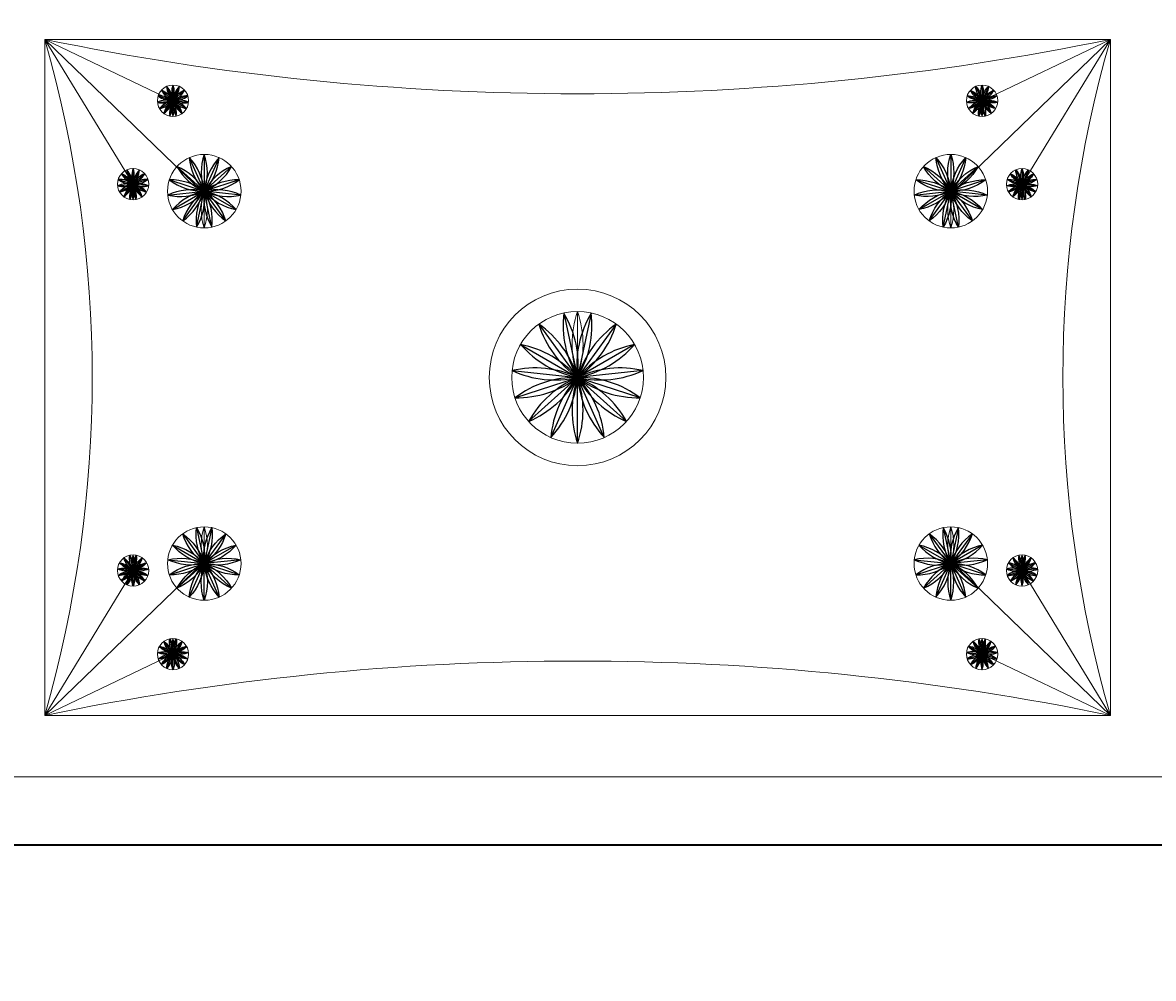
# Model space of a CAD drawing. Units: inches. Extents: x -61 to 1599, y -1316 to 257.
# Tile 115 of 204: x 109 to 134, y -10 to 11. Entities that reach past the tile are written whole.
import ezdxf

# ---------------------------------------------------------------- set-up
doc = ezdxf.new("R2010")
doc.units = ezdxf.units.IN
doc.header["$MEASUREMENT"] = 0
for name, color, linetype, lineweight in [('A-ANNO-DIMS', 2, 'Continuous', 18), ('FURNITURE', 83, 'Continuous', 18), ('WALLS', 4, 'Continuous', 35)]:
    doc.layers.add(name, color=color, linetype=linetype, lineweight=lineweight)
doc.layers.add('LT', color=8, linetype='Continuous')
doc.styles.get("Standard").update_dxf_attribs({"font": 'arial.ttf'})
doc.dimstyles.get("Standard").update_dxf_attribs({"dimtxt": 0.18, "dimasz": 0.18, "dimexe": 0.18, "dimexo": 0.0625, "dimgap": 0.09, "dimtad": 0, "dimtih": 1, "dimtoh": 1, "dimdec": 0, "dimzin": 0, "dimdsep": 46, "dimlunit": 3, "dimtxsty": 'Standard', "dimcen": 0.09, "dimadec": 0, "dimazin": 0, "dimtfac": 1, "dimtdec": 0, "dimtofl": 0, "dimtmove": 0, "dimatfit": 3, "dimfxl": 1, "dimtolj": 1, "dimtzin": 0, "dimarcsym": 0})

# ---------------------------------------------------------------- blocks, each defined once
blk = doc.blocks.new('*U15')
at = {"layer": 'LT'}
blk.add_line((0, 0.175), (0, -0.175), dxfattribs=at)
for centre, start, end in [((0.509, 0), 160.9983, 199.0017), ((-0.509, 0), 340.9983, 19.0017)]:
    blk.add_arc(centre, 0.539, start, end, dxfattribs=at)
blk = doc.blocks.new('*U16')
at = {"layer": 'LT', "transparency": 16777216}
for p, rotation in [((-66.546, -18.649), 24), ((-66.404, -18.649), 336.0000000000001), ((-66.642, -18.755), 72), ((-66.605, -18.692), 48.00000000000001), ((-66.345, -18.692), 312), ((-66.308, -18.755), 288.0000000000001), ((-66.649, -18.828), 96), ((-66.627, -18.897), 120), ((-66.578, -18.951), 144), ((-66.512, -18.981), 168.0000000000001), ((-66.439, -18.981), 192), ((-66.372, -18.951), 216), ((-66.323, -18.897), 240), ((-66.301, -18.828), 264)]:
    blk.add_blockref('*U15', p, dxfattribs=dict(at, rotation=rotation))
blk.add_blockref('*U15', (-66.475, -18.634), dxfattribs=at)
blk = doc.blocks.new('*U45')
at = {"layer": 'LT'}
blk.add_line((0, 0.175), (0, -0.175), dxfattribs=at)
for centre, start, end in [((0.509, 0), 160.9983, 199.0017), ((-0.509, 0), 340.9983, 19.0017)]:
    blk.add_arc(centre, 0.539, start, end, dxfattribs=at)
blk = doc.blocks.new('*U46')
at = {"layer": 'LT', "transparency": 16777216}
for p, rotation in [((-66.546, -18.649), 24), ((-66.404, -18.649), 336.0000000000001), ((-66.642, -18.755), 72), ((-66.605, -18.692), 48.00000000000001), ((-66.345, -18.692), 312), ((-66.308, -18.755), 288.0000000000001), ((-66.649, -18.828), 96), ((-66.627, -18.897), 120), ((-66.578, -18.951), 144), ((-66.512, -18.981), 168.0000000000001), ((-66.439, -18.981), 192), ((-66.372, -18.951), 216), ((-66.323, -18.897), 240), ((-66.301, -18.828), 264)]:
    blk.add_blockref('*U45', p, dxfattribs=dict(at, rotation=rotation))
blk.add_blockref('*U45', (-66.475, -18.634), dxfattribs=at)
blk = doc.blocks.new('*U9')
at = {"layer": 'LT'}
blk.add_line((0, 0.175), (0, -0.175), dxfattribs=at)
for centre, start, end in [((0.509, 0), 160.9983, 199.0017), ((-0.509, 0), 340.9983, 19.0017)]:
    blk.add_arc(centre, 0.539, start, end, dxfattribs=at)
blk = doc.blocks.new('*U10')
at = {"layer": 'LT', "transparency": 16777216}
for p, rotation in [((-66.546, -18.649), 24), ((-66.404, -18.649), 336.0000000000001), ((-66.642, -18.755), 72), ((-66.605, -18.692), 48.00000000000001), ((-66.345, -18.692), 312), ((-66.308, -18.755), 288.0000000000001), ((-66.649, -18.828), 96), ((-66.627, -18.897), 120), ((-66.578, -18.951), 144), ((-66.512, -18.981), 168.0000000000001), ((-66.439, -18.981), 192), ((-66.372, -18.951), 216), ((-66.323, -18.897), 240), ((-66.301, -18.828), 264)]:
    blk.add_blockref('*U9', p, dxfattribs=dict(at, rotation=rotation))
blk.add_blockref('*U9', (-66.475, -18.634), dxfattribs=at)
blk = doc.blocks.new('*U39')
at = {"layer": 'LT'}
blk.add_line((0, 0.175), (0, -0.175), dxfattribs=at)
for centre, start, end in [((0.509, 0), 160.9983, 199.0017), ((-0.509, 0), 340.9983, 19.0017)]:
    blk.add_arc(centre, 0.539, start, end, dxfattribs=at)
blk = doc.blocks.new('*U40')
at = {"layer": 'LT', "transparency": 16777216}
for p, rotation in [((-66.546, -18.649), 24), ((-66.404, -18.649), 336.0000000000001), ((-66.642, -18.755), 72), ((-66.605, -18.692), 48.00000000000001), ((-66.345, -18.692), 312), ((-66.308, -18.755), 288.0000000000001), ((-66.649, -18.828), 96), ((-66.627, -18.897), 120), ((-66.578, -18.951), 144), ((-66.512, -18.981), 168.0000000000001), ((-66.439, -18.981), 192), ((-66.372, -18.951), 216), ((-66.323, -18.897), 240), ((-66.301, -18.828), 264)]:
    blk.add_blockref('*U39', p, dxfattribs=dict(at, rotation=rotation))
blk.add_blockref('*U39', (-66.475, -18.634), dxfattribs=at)
blk = doc.blocks.new('*U17')
at = {"layer": 'LT'}
blk.add_line((0, 0.412), (0, -0.412), dxfattribs=at)
for centre, start, end in [((1.198, 0), 160.9983, 199.0017), ((-1.198, 0), 340.9983, 19.0017)]:
    blk.add_arc(centre, 1.267, start, end, dxfattribs=at)
blk = doc.blocks.new('*U18')
at = {"layer": 'LT', "transparency": 16777216}
for p, rotation in [((-156.639, -43.959), 48.00000000000001), ((-156.501, -43.858), 24), ((-156.165, -43.858), 336.0000000000001), ((-156.027, -43.959), 312), ((-156.725, -44.108), 72), ((-155.941, -44.108), 288.0000000000001), ((-156.743, -44.278), 96), ((-156.69, -44.441), 120), ((-156.575, -44.569), 144), ((-156.419, -44.639), 168), ((-156.247, -44.639), 192), ((-156.091, -44.569), 216), ((-155.976, -44.441), 240), ((-155.923, -44.278), 264)]:
    blk.add_blockref('*U17', p, dxfattribs=dict(at, rotation=rotation))
blk.add_blockref('*U17', (-156.333, -43.823), dxfattribs=at)
blk = doc.blocks.new('*U33')
at = {"layer": 'LT'}
blk.add_line((0, 0.412), (0, -0.412), dxfattribs=at)
for centre, start, end in [((1.198, 0), 160.9983, 199.0017), ((-1.198, 0), 340.9983, 19.0017)]:
    blk.add_arc(centre, 1.267, start, end, dxfattribs=at)
blk = doc.blocks.new('*U34')
at = {"layer": 'LT', "transparency": 16777216}
for p, rotation in [((-156.639, -43.959), 48.00000000000001), ((-156.501, -43.858), 24), ((-156.165, -43.858), 336.0000000000001), ((-156.027, -43.959), 312), ((-156.725, -44.108), 72), ((-155.941, -44.108), 288.0000000000001), ((-156.743, -44.278), 96), ((-156.69, -44.441), 120), ((-156.575, -44.569), 144), ((-156.419, -44.639), 168), ((-156.247, -44.639), 192), ((-156.091, -44.569), 216), ((-155.976, -44.441), 240), ((-155.923, -44.278), 264)]:
    blk.add_blockref('*U33', p, dxfattribs=dict(at, rotation=rotation))
blk.add_blockref('*U33', (-156.333, -43.823), dxfattribs=at)
blk = doc.blocks.new('*U11')
at = {"layer": 'LT'}
blk.add_line((0, 0.739), (0, -0.739), dxfattribs=at)
for centre, start, end in [((2.147, 0), 160.9983, 199.0017), ((-2.147, 0), 340.9983, 19.0017)]:
    blk.add_arc(centre, 2.27, start, end, dxfattribs=at)
blk = doc.blocks.new('*U12')
at = {"layer": 'LT', "transparency": 16777216}
for p, rotation in [((-280.542, -78.621), 23.99999999999999), ((-279.941, -78.621), 336.0000000000001), ((-280.791, -78.801), 48.00000000000001), ((-279.692, -78.801), 312), ((-280.945, -79.067), 72), ((-279.539, -79.067), 288.0000000000001), ((-280.977, -79.373), 96), ((-279.507, -79.373), 264), ((-280.882, -79.665), 120), ((-280.676, -79.894), 144), ((-280.395, -80.019), 168), ((-280.088, -80.019), 191.9999999999999), ((-279.807, -79.894), 216), ((-279.602, -79.665), 240)]:
    blk.add_blockref('*U11', p, dxfattribs=dict(at, rotation=rotation))
blk.add_blockref('*U11', (-280.242, -78.557), dxfattribs=at)
blk = doc.blocks.new('*U28')
at = {"layer": 'LT'}
blk.add_line((0, 0.412), (0, -0.412), dxfattribs=at)
for centre, start, end in [((1.198, 0), 160.9983, 199.0017), ((-1.198, 0), 340.9983, 19.0017)]:
    blk.add_arc(centre, 1.267, start, end, dxfattribs=at)
blk = doc.blocks.new('*U44')
at = {"layer": 'LT', "transparency": 16777216}
for p, rotation in [((-156.639, -43.959), 48.00000000000001), ((-156.501, -43.858), 24), ((-156.165, -43.858), 336.0000000000001), ((-156.027, -43.959), 312), ((-156.725, -44.108), 72), ((-155.941, -44.108), 288.0000000000001), ((-156.743, -44.278), 96), ((-156.69, -44.441), 120), ((-156.575, -44.569), 144), ((-156.419, -44.639), 168), ((-156.247, -44.639), 192), ((-156.091, -44.569), 216), ((-155.976, -44.441), 240), ((-155.923, -44.278), 264)]:
    blk.add_blockref('*U28', p, dxfattribs=dict(at, rotation=rotation))
blk.add_blockref('*U28', (-156.333, -43.823), dxfattribs=at)
blk = doc.blocks.new('*U13')
at = {"layer": 'LT'}
blk.add_line((0, 0.412), (0, -0.412), dxfattribs=at)
for centre, start, end in [((1.198, 0), 160.9983, 199.0017), ((-1.198, 0), 340.9983, 19.0017)]:
    blk.add_arc(centre, 1.267, start, end, dxfattribs=at)
blk = doc.blocks.new('*U14')
at = {"layer": 'LT', "transparency": 16777216}
for p, rotation in [((-156.639, -43.959), 48.00000000000001), ((-156.501, -43.858), 24), ((-156.165, -43.858), 336.0000000000001), ((-156.027, -43.959), 312), ((-156.725, -44.108), 72), ((-155.941, -44.108), 288.0000000000001), ((-156.743, -44.278), 96), ((-156.69, -44.441), 120), ((-156.575, -44.569), 144), ((-156.419, -44.639), 168), ((-156.247, -44.639), 192), ((-156.091, -44.569), 216), ((-155.976, -44.441), 240), ((-155.923, -44.278), 264)]:
    blk.add_blockref('*U13', p, dxfattribs=dict(at, rotation=rotation))
blk.add_blockref('*U13', (-156.333, -43.823), dxfattribs=at)
blk = doc.blocks.new('*U19')
at = {"layer": 'LT'}
blk.add_line((0, 0.175), (0, -0.175), dxfattribs=at)
for centre, start, end in [((0.509, 0), 160.9983, 199.0017), ((-0.509, 0), 340.9983, 19.0017)]:
    blk.add_arc(centre, 0.539, start, end, dxfattribs=at)
blk = doc.blocks.new('*U6')
at = {"layer": 'LT', "transparency": 16777216}
for p, rotation in [((-66.546, -18.649), 24), ((-66.404, -18.649), 336.0000000000001), ((-66.642, -18.755), 72), ((-66.605, -18.692), 48.00000000000001), ((-66.345, -18.692), 312), ((-66.308, -18.755), 288.0000000000001), ((-66.649, -18.828), 96), ((-66.627, -18.897), 120), ((-66.578, -18.951), 144), ((-66.512, -18.981), 168.0000000000001), ((-66.439, -18.981), 192), ((-66.372, -18.951), 216), ((-66.323, -18.897), 240), ((-66.301, -18.828), 264)]:
    blk.add_blockref('*U19', p, dxfattribs=dict(at, rotation=rotation))
blk.add_blockref('*U19', (-66.475, -18.634), dxfattribs=at)
blk = doc.blocks.new('*U35')
at = {"layer": 'LT'}
blk.add_line((0, 0.175), (0, -0.175), dxfattribs=at)
for centre, start, end in [((0.509, 0), 160.9983, 199.0017), ((-0.509, 0), 340.9983, 19.0017)]:
    blk.add_arc(centre, 0.539, start, end, dxfattribs=at)
blk = doc.blocks.new('*U36')
at = {"layer": 'LT', "transparency": 16777216}
for p, rotation in [((-66.546, -18.649), 24), ((-66.404, -18.649), 336.0000000000001), ((-66.642, -18.755), 72), ((-66.605, -18.692), 48.00000000000001), ((-66.345, -18.692), 312), ((-66.308, -18.755), 288.0000000000001), ((-66.649, -18.828), 96), ((-66.627, -18.897), 120), ((-66.578, -18.951), 144), ((-66.512, -18.981), 168.0000000000001), ((-66.439, -18.981), 192), ((-66.372, -18.951), 216), ((-66.323, -18.897), 240), ((-66.301, -18.828), 264)]:
    blk.add_blockref('*U35', p, dxfattribs=dict(at, rotation=rotation))
blk.add_blockref('*U35', (-66.475, -18.634), dxfattribs=at)
blk = doc.blocks.new('*U7')
at = {"layer": 'LT'}
blk.add_line((0, 0.175), (0, -0.175), dxfattribs=at)
for centre, start, end in [((0.509, 0), 160.9983, 199.0017), ((-0.509, 0), 340.9983, 19.0017)]:
    blk.add_arc(centre, 0.539, start, end, dxfattribs=at)
blk = doc.blocks.new('*U8')
at = {"layer": 'LT', "transparency": 16777216}
for p, rotation in [((-66.546, -18.649), 24), ((-66.404, -18.649), 336.0000000000001), ((-66.642, -18.755), 72), ((-66.605, -18.692), 48.00000000000001), ((-66.345, -18.692), 312), ((-66.308, -18.755), 288.0000000000001), ((-66.649, -18.828), 96), ((-66.627, -18.897), 120), ((-66.578, -18.951), 144), ((-66.512, -18.981), 168.0000000000001), ((-66.439, -18.981), 192), ((-66.372, -18.951), 216), ((-66.323, -18.897), 240), ((-66.301, -18.828), 264)]:
    blk.add_blockref('*U7', p, dxfattribs=dict(at, rotation=rotation))
blk.add_blockref('*U7', (-66.475, -18.634), dxfattribs=at)
blk = doc.blocks.new('*U37')
at = {"layer": 'LT'}
blk.add_line((0, 0.175), (0, -0.175), dxfattribs=at)
for centre, start, end in [((0.509, 0), 160.9983, 199.0017), ((-0.509, 0), 340.9983, 19.0017)]:
    blk.add_arc(centre, 0.539, start, end, dxfattribs=at)
blk = doc.blocks.new('*U38')
at = {"layer": 'LT', "transparency": 16777216}
for p, rotation in [((-66.546, -18.649), 24), ((-66.404, -18.649), 336.0000000000001), ((-66.642, -18.755), 72), ((-66.605, -18.692), 48.00000000000001), ((-66.345, -18.692), 312), ((-66.308, -18.755), 288.0000000000001), ((-66.649, -18.828), 96), ((-66.627, -18.897), 120), ((-66.578, -18.951), 144), ((-66.512, -18.981), 168.0000000000001), ((-66.439, -18.981), 192), ((-66.372, -18.951), 216), ((-66.323, -18.897), 240), ((-66.301, -18.828), 264)]:
    blk.add_blockref('*U37', p, dxfattribs=dict(at, rotation=rotation))
blk.add_blockref('*U37', (-66.475, -18.634), dxfattribs=at)
blk = doc.blocks.new('BED-DOUBLE')
for p, q in [((10.471, 1.379), (10.471, 16.557)), ((34.388, 16.557), (10.471, 16.557)), ((10.471, 16.557), (13.35, 15.18)), ((10.471, 16.557), (14.039, 13.107)), ((10.471, 16.557), (12.454, 13.305)), ((34.388, 16.557), (30.82, 13.107)), ((34.388, 16.557), (31.508, 15.18)), ((34.388, 16.557), (32.405, 13.305)), ((13.35, 15.18), (13.35, 14.829)), ((31.508, 15.18), (31.508, 14.829)), ((12.454, 13.305), (12.454, 12.955)), ((32.405, 13.305), (32.405, 12.955)), ((14.052, 13.149), (14.052, 12.324)), ((30.806, 13.149), (30.806, 12.324)), ((22.429, 8.968), (22.429, 10.447)), ((14.052, 4.788), (14.052, 5.613)), ((30.806, 4.788), (30.806, 5.613)), ((10.471, 1.379), (14.039, 4.83)), ((12.454, 4.631), (12.454, 4.982)), ((34.388, 1.379), (30.82, 4.83)), ((32.405, 4.631), (32.405, 4.982)), ((10.471, 1.379), (12.454, 4.631)), ((34.388, 1.379), (32.405, 4.631)), ((13.35, 2.756), (13.35, 3.107)), ((31.508, 2.756), (31.508, 3.107)), ((10.471, 1.379), (13.35, 2.756)), ((34.388, 1.379), (31.508, 2.756)), ((34.388, 1.379), (34.388, 1.379))]:
    blk.add_line(p, q)
for points in [[(1.272, 88.537), (1.272, 3.449, 0.414214), (4.722, 0), (66.813, 0, 0.414214), (70.263, 3.449), (70.263, 88.537, 0.414214), (66.813, 91.987), (4.722, 91.987, 0.414214)], [(13.35, 15.18, 0.167358), (13.35, 14.829, 0.167358)], [(12.454, 13.305, 0.167358), (12.454, 12.955, 0.167358)], [(32.405, 12.955, 0.167358), (32.405, 13.305, 0.167358)], [(14.052, 13.149, 0.167358), (14.052, 12.324, 0.167358)], [(30.806, 12.324, 0.167358), (30.806, 13.149, 0.167358)], [(22.429, 8.968, 0.167358), (22.429, 10.447, 0.167358)], [(14.052, 5.613, 0.167358), (14.052, 4.788, 0.167358)], [(30.806, 4.788, 0.167358), (30.806, 5.613, 0.167358)], [(12.454, 4.982, 0.167358), (12.454, 4.631, 0.167358)], [(32.405, 4.631, 0.167358), (32.405, 4.982, 0.167358)], [(13.35, 3.107, 0.167358), (13.35, 2.756, 0.167358)], [(31.508, 2.756, 0.167358), (31.508, 3.107, 0.167358)]]:
    blk.add_lwpolyline(points, format="xyb", close=True)
blk.add_lwpolyline([(34.388, 16.557), (34.388, 1.379), (10.471, 1.379), (10.471, 16.557), (34.388, 16.557), (34.388, 1.379), (10.471, 1.379)])
for centre, radius in [((13.35, 15.18), 0.351), ((31.508, 15.18), 0.351), ((14.052, 13.149), 0.825), ((30.806, 13.149), 0.825), ((12.454, 13.305), 0.351), ((32.405, 13.305), 0.351), ((22.429, 8.968), 1.982), ((22.429, 8.968), 1.478), ((14.052, 4.788), 0.825), ((30.806, 4.788), 0.825), ((12.454, 4.631), 0.351), ((32.405, 4.631), 0.351), ((13.35, 2.756), 0.351), ((31.508, 2.756), 0.351)]:
    blk.add_circle(centre, radius)
for centre, radius, start, end in [((-16.003, 8.968), 27.54, 344.0046, 15.9954), ((22.429, 74.54), 59.203, 258.34678, 281.65322), ((60.861, 8.968), 27.54, 164.0046, 195.9954), ((32.017, 15.005), 0.539, 160.9983, 199.0017), ((30.999, 15.005), 0.539, 340.9983, 19.0017), ((22.429, -56.603), 59.203, 78.34678, 101.65322)]:
    blk.add_arc(centre, radius, start, end)
for name, p in [('*U40', (79.825, 33.99)), ('*U34', (170.385, 57.384)), ('*U46', (78.929, 32.115))]:
    blk.add_blockref(name, p)
at = {"extrusion": (0, 0, -1), "zscale": -1}
for name, p in [('*U36', (34.967, 33.99)), ('*U14', (125.527, 57.384)), ('*U38', (34.07, 32.115))]:
    blk.add_blockref(name, p, dxfattribs=at)
at = {"rotation": 180}
for name, p in [('*U12', (-257.812, -70.328)), ('*U44', (-125.527, -39.447)), ('*U8', (-34.07, -14.178)), ('*U6', (-34.967, -16.053))]:
    blk.add_blockref(name, p, dxfattribs=at)
at = {"extrusion": (0, 0, -1), "zscale": -1, "rotation": 180}
for name, p in [('*U18', (-170.385, -39.447)), ('*U16', (-78.929, -14.178)), ('*U10', (-79.825, -16.053))]:
    blk.add_blockref(name, p, dxfattribs=at)
blk = doc.blocks.new('*D687')
at = {"layer": 'A-ANNO-DIMS', "color": 0, "lineweight": -2, "transparency": 16777216}
for p, q in [((289.418, 181.677), (-61.077, 181.677)), ((-60.897, 181.497), (-60.897, -528.952)), ((-60.897, -1239.765), (-60.897, -529.316)), ((319.64, -1239.945), (-61.077, -1239.945))]:
    blk.add_line(p, q, dxfattribs=at)
at = {"layer": 'A-ANNO-DIMS', "color": 0, "transparency": 16777216}
for points in [[(-60.927, 181.497), (-60.867, 181.497), (-60.897, 181.677)], [(-60.927, -1239.765), (-60.867, -1239.765), (-60.897, -1239.945)]]:
    blk.add_solid(points, dxfattribs=at)
at = {"layer": 'DEFPOINTS', "color": 0, "transparency": 16777216}
for p in [(289.481, 181.677), (-60.897, -1239.945), (319.703, -1239.945)]:
    blk.add_point(p, dxfattribs=at)
at = {"layer": 'A-ANNO-DIMS', "color": 0, "transparency": 16777216, "insert": (-60.897, -529.134), "char_height": 0.18, "attachment_point": 5}
blk.add_mtext('\\A1;1421.6', dxfattribs=at)
blk = doc.blocks.new('*D700')
at = {"layer": 'A-ANNO-DIMS', "color": 0, "lineweight": -2, "transparency": 16777216}
for p, q in [((14.703, -616.882), (14.703, 257.457)), ((179.752, -616.882), (179.752, 257.457)), ((14.883, 257.277), (96.772, 257.277)), ((179.572, 257.277), (97.683, 257.277))]:
    blk.add_line(p, q, dxfattribs=at)
at = {"layer": 'A-ANNO-DIMS', "color": 0, "transparency": 16777216}
for points in [[(14.883, 257.307), (14.883, 257.247), (14.703, 257.277)], [(179.572, 257.307), (179.572, 257.247), (179.752, 257.277)]]:
    blk.add_solid(points, dxfattribs=at)
at = {"layer": 'DEFPOINTS', "color": 0, "transparency": 16777216}
for p in [(179.752, 257.277), (14.703, -616.945), (179.752, -616.945)]:
    blk.add_point(p, dxfattribs=at)
at = {"layer": 'A-ANNO-DIMS', "color": 0, "transparency": 16777216, "insert": (97.227, 257.277), "char_height": 0.18, "attachment_point": 5}
blk.add_mtext('\\A1;165.05', dxfattribs=at)

msp = doc.modelspace()

# ---------------------------------------------------------------- linework, layer by layer
at = {"layer": 'WALLS'}
msp.add_line((87.7028, -7.3229), (185.2611, -7.3229), dxfattribs=at)

# ---------------------------------------------------------------- block references
at = {"layer": 'FURNITURE'}
msp.add_blockref('BED-DOUBLE', (98.977, -5.797), dxfattribs=at)

# ---------------------------------------------------------------- dimensions: what is measured, and where the dimension line sits
at = {"layer": 'A-ANNO-DIMS'}
dim = msp.add_linear_dim(base=(179.7521, 257.2771), p1=(14.7028, -616.9446), p2=(179.7521, -616.9446), dimstyle='Standard', override={"dimdec": 2, "dimlfac": 1, "dimrnd": 0, "dimzin": 0, "dimdsep": 46, "dimlunit": 2}, dxfattribs=at)
dim.commit()
dim.dimension.update_dxf_attribs({"geometry": '*D700', "text_midpoint": (97.2274, 257.2771)})
dim = msp.add_linear_dim(base=(-60.8972, -1239.9446), p1=(289.4807, 181.6771), p2=(319.7028, -1239.9446), angle=90, dimstyle='Standard', override={"dimdec": 1, "dimlfac": 1, "dimrnd": 0, "dimzin": 0, "dimdsep": 46, "dimlunit": 2}, dxfattribs=at)
dim.commit()
dim.dimension.update_dxf_attribs({"geometry": '*D687', "text_midpoint": (-60.8972, -529.1337)})

doc.saveas('drawing.dxf')
